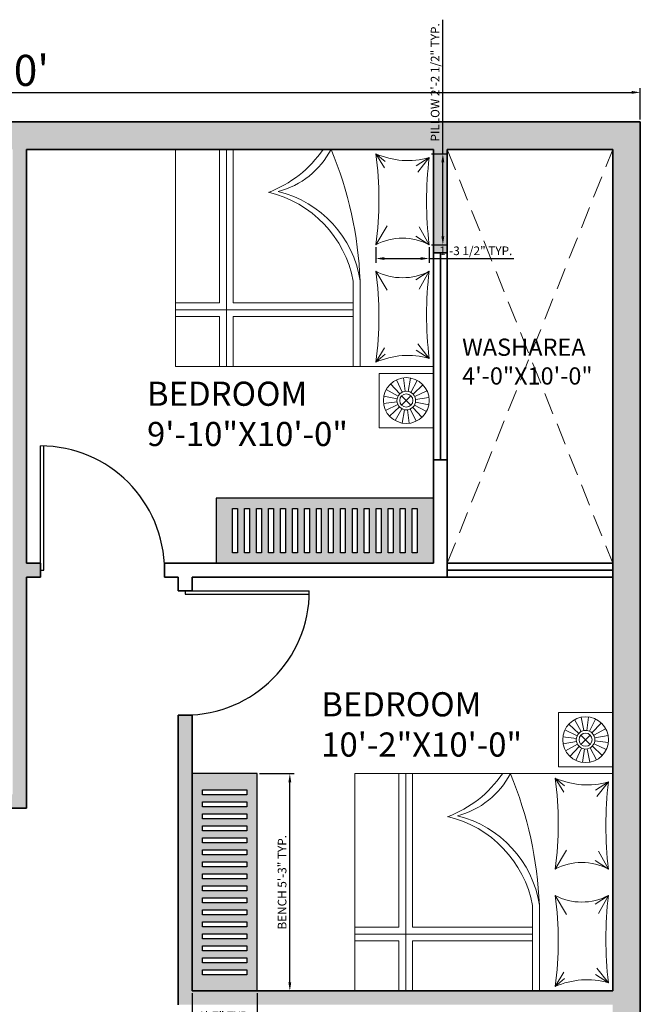
# Model space of a CAD drawing. Units: inches. Extents: x 1566 to 2546, y 1087 to 2705.
# Tile 23 of 27: x 2278 to 2458, y 1529 to 1814. Entities that reach past the tile are written whole.
import ezdxf

# ---------------------------------------------------------------- set-up
doc = ezdxf.new("R2010")
doc.units = ezdxf.units.IN
doc.linetypes.add('DASHED', pattern=[19.05, 12.7, -6.35])
for name, color, linetype, lineweight in [('A-ANNO-DIMS', 2, 'Continuous', 18), ('A-AREA-IDEN', 7, 'Continuous', 18), ('A-DOOR', 4, 'Continuous', 25), ('A-FLOR-OVHD', 8, 'DASHED', 18), ('A-FURN', 8, 'Continuous', 18), ('A-WALL', 7, 'Continuous', 35), ('A-WALL-PATT', 8, 'Continuous', 13)]:
    doc.layers.add(name, color=color, linetype=linetype, lineweight=lineweight)
doc.layers.add('MESA', color=7, linetype='Continuous')
doc.styles.get("Standard").update_dxf_attribs({"font": 'arial.ttf'})
doc.dimstyles.new('ISO-25', dxfattribs={"dimtxt": 2.5, "dimasz": 2.5, "dimexe": 1.25, "dimexo": 0.625, "dimtad": 1, "dimtxsty": 'Standard', "dimcen": 2.5, "dimadec": 0, "dimazin": 0, "dimtfac": 1, "dimtmove": 0, "dimatfit": 3, "dimfxl": 1, "dimarcsym": 0})

# ---------------------------------------------------------------- blocks, each defined once
blk = doc.blocks.new('*D2')
at = {"layer": 'A-ANNO-DIMS', "color": 0, "lineweight": -2, "transparency": 16777216}
for p, q in [((2098.29, 1785.06), (2098.29, 1794.2)), ((2100.79, 1792.95), (2455.79, 1792.95)), ((2458.29, 1785.06), (2458.29, 1794.2))]:
    blk.add_line(p, q, dxfattribs=at)
at = {"layer": 'A-ANNO-DIMS', "color": 0, "transparency": 16777216}
for points in [[(2100.79, 1793.37), (2100.79, 1792.53), (2098.29, 1792.95)], [(2455.79, 1793.37), (2455.79, 1792.53), (2458.29, 1792.95)]]:
    blk.add_solid(points, dxfattribs=at)
at = {"layer": 'Defpoints', "color": 0, "transparency": 16777216}
for p in [(2458.29, 1792.95), (2098.29, 1784.43), (2458.29, 1784.43)]:
    blk.add_point(p, dxfattribs=at)
at = {"layer": 'A-ANNO-DIMS', "color": 0, "transparency": 16777216, "insert": (2278.29, 1798.17), "char_height": 9, "attachment_point": 5}
blk.add_mtext("30'", dxfattribs=at)
blk = doc.blocks.new('d1')
for p, q in [((3297.32, 1596.93), (3297.32, 1632.93)), ((3298.32, 1596.93), (3298.32, 1632.93)), ((3297.32, 1596.93), (3298.32, 1596.93))]:
    blk.add_line(p, q)
at = {"ltscale": 0.3}
blk.add_arc((3297.32, 1596.93), 36, 0, 90, dxfattribs=at)
blk = doc.blocks.new('Banco Lintz')
at = {"layer": 'MESA', "ltscale": 0.05}
h = blk.add_hatch(color=256, dxfattribs=at)
h.dxf.hatch_style = 1
h.set_gradient(color1=(138, 84, 66), color2=(0, 0, 0), one_color=1, name='INVCYLINDER')
h.paths.add_polyline_path([(0.48, 0), (0, 0), (0, -1.6), (0.48, -1.6)])
h.paths.add_polyline_path([(0.4034, -0.5091), (0.0766, -0.5091), (0.0766, -0.4724), (0.4034, -0.4724)], flags=16)
h.paths.add_polyline_path([(0.4034, -0.5608), (0.4034, -0.5974), (0.0766, -0.5974), (0.0766, -0.5608)], flags=16)
h.paths.add_polyline_path([(0.4034, -0.4207), (0.0766, -0.4207), (0.0766, -0.384), (0.4034, -0.384)], flags=16)
h.paths.add_polyline_path([(0.4034, -0.6491), (0.4034, -0.6858), (0.0766, -0.6858), (0.0766, -0.6491)], flags=16)
h.paths.add_polyline_path([(0.4034, -0.3323), (0.0766, -0.3323), (0.0766, -0.2957), (0.4034, -0.2957)], flags=16)
h.paths.add_polyline_path([(0.4034, -0.7375), (0.4034, -0.7741), (0.0766, -0.7741), (0.0766, -0.7375)], flags=16)
h.paths.add_polyline_path([(0.4034, -0.244), (0.0766, -0.244), (0.0766, -0.2073), (0.4034, -0.2073)], flags=16)
h.paths.add_polyline_path([(0.4034, -0.8259), (0.4034, -0.8625), (0.0766, -0.8625), (0.0766, -0.8259)], flags=16)
h.paths.add_polyline_path([(0.4034, -0.1556), (0.0766, -0.1556), (0.0766, -0.119), (0.4034, -0.119)], flags=16)
h.paths.add_polyline_path([(0.4034, -0.9142), (0.4034, -0.9509), (0.0766, -0.9509), (0.0766, -0.9142)], flags=16)
h.paths.add_polyline_path([(0.4034, -1.0026), (0.4034, -1.0392), (0.0766, -1.0392), (0.0766, -1.0026)], flags=16)
h.paths.add_polyline_path([(0.4034, -1.0909), (0.4034, -1.1276), (0.0766, -1.1276), (0.0766, -1.0909)], flags=16)
h.paths.add_polyline_path([(0.4034, -1.1793), (0.4034, -1.216), (0.0766, -1.216), (0.0766, -1.1793)], flags=16)
h.paths.add_polyline_path([(0.4034, -1.2677), (0.4034, -1.3043), (0.0766, -1.3043), (0.0766, -1.2677)], flags=16)
h.paths.add_polyline_path([(0.4034, -1.356), (0.4034, -1.3927), (0.0766, -1.3927), (0.0766, -1.356)], flags=16)
h.paths.add_polyline_path([(0.4034, -1.4444), (0.4034, -1.481), (0.0766, -1.481), (0.0766, -1.4444)], flags=16)
for points in [[(0, -1.6), (0.48, -1.6), (0.48, 0), (0, 0)], [(0.0766, -0.119), (0.4034, -0.119), (0.4034, -0.1556), (0.0766, -0.1556)], [(0.0766, -0.2073), (0.4034, -0.2073), (0.4034, -0.244), (0.0766, -0.244)], [(0.0766, -0.2957), (0.4034, -0.2957), (0.4034, -0.3323), (0.0766, -0.3323)], [(0.0766, -0.384), (0.4034, -0.384), (0.4034, -0.4207), (0.0766, -0.4207)], [(0.0766, -0.4724), (0.4034, -0.4724), (0.4034, -0.5091), (0.0766, -0.5091)], [(0.0766, -0.5608), (0.4034, -0.5608), (0.4034, -0.5974), (0.0766, -0.5974)], [(0.0766, -0.6491), (0.4034, -0.6491), (0.4034, -0.6858), (0.0766, -0.6858)], [(0.0766, -0.7375), (0.4034, -0.7375), (0.4034, -0.7741), (0.0766, -0.7741)], [(0.0766, -0.8259), (0.4034, -0.8259), (0.4034, -0.8625), (0.0766, -0.8625)], [(0.0766, -0.9142), (0.4034, -0.9142), (0.4034, -0.9509), (0.0766, -0.9509)], [(0.0766, -1.0026), (0.4034, -1.0026), (0.4034, -1.0392), (0.0766, -1.0392)], [(0.0766, -1.0909), (0.4034, -1.0909), (0.4034, -1.1276), (0.0766, -1.1276)], [(0.0766, -1.1793), (0.4034, -1.1793), (0.4034, -1.216), (0.0766, -1.216)], [(0.0766, -1.2677), (0.4034, -1.2677), (0.4034, -1.3043), (0.0766, -1.3043)], [(0.0766, -1.356), (0.4034, -1.356), (0.4034, -1.3927), (0.0766, -1.3927)], [(0.0766, -1.4444), (0.4034, -1.4444), (0.4034, -1.481), (0.0766, -1.481)]]:
    blk.add_lwpolyline(points, close=True, dxfattribs=at)
blk = doc.blocks.new('PILLOW')
for p, q in [((0, 26.42), (2.52, 22.29)), ((0, 26.42), (2.72, 24.12)), ((15.48, 25.29), (11.7, 22.89)), ((15.48, 25.29), (12.15, 21.04)), ((0, 0), (3.27, 5.54)), ((15.48, 0), (12.59, 5.2)), ((15.48, 0), (11.65, 2.52))]:
    blk.add_line(p, q)
for points in [[(0, 26.42, -0.069628), (0, 0)], [(0, 26.42, 0.175461), (15.48, 25.29)], [(15.48, 25.29, 0.059544), (15.48, 0)], [(0, 0, -0.248743), (15.48, 0)]]:
    blk.add_lwpolyline(points, format="xyb")
blk = doc.blocks.new('*D41')
at = {"layer": 'A-ANNO-DIMS', "color": 0, "lineweight": -2, "transparency": 16777216}
for p, q in [((2347.81, 1595.43), (2357.89, 1595.43)), ((2356.64, 1534.93), (2356.64, 1592.93)), ((2347.81, 1532.43), (2357.89, 1532.43))]:
    blk.add_line(p, q, dxfattribs=at)
at = {"layer": 'A-ANNO-DIMS', "color": 0, "transparency": 16777216}
for points in [[(2356.22, 1592.93), (2357.05, 1592.93), (2356.64, 1595.43)], [(2356.22, 1534.93), (2357.05, 1534.93), (2356.64, 1532.43)]]:
    blk.add_solid(points, dxfattribs=at)
at = {"layer": 'Defpoints', "color": 0, "transparency": 16777216}
for p in [(2347.19, 1595.43), (2356.64, 1595.43), (2347.19, 1532.43)]:
    blk.add_point(p, dxfattribs=at)
at = {"layer": 'A-ANNO-DIMS', "color": 0, "transparency": 16777216, "insert": (2354.72, 1563.93), "char_height": 2.5, "attachment_point": 5, "rotation": 90}
blk.add_mtext('BENCH 5\'-3" TYP.', dxfattribs=at)
blk = doc.blocks.new('*D42')
at = {"layer": 'A-ANNO-DIMS', "color": 0, "lineweight": -2, "transparency": 16777216}
for p, q in [((2328.29, 1531.81), (2328.29, 1521.73)), ((2347.19, 1531.81), (2347.19, 1521.73)), ((2330.79, 1522.98), (2344.69, 1522.98))]:
    blk.add_line(p, q, dxfattribs=at)
at = {"layer": 'A-ANNO-DIMS', "color": 0, "transparency": 16777216}
for points in [[(2330.79, 1523.4), (2330.79, 1522.57), (2328.29, 1522.98)], [(2344.69, 1523.4), (2344.69, 1522.57), (2347.19, 1522.98)]]:
    blk.add_solid(points, dxfattribs=at)
at = {"layer": 'Defpoints', "color": 0, "transparency": 16777216}
for p in [(2328.29, 1532.43), (2347.19, 1532.43), (2347.19, 1522.98)]:
    blk.add_point(p, dxfattribs=at)
at = {"layer": 'A-ANNO-DIMS', "color": 0, "transparency": 16777216, "insert": (2337.74, 1524.87), "char_height": 2.5, "attachment_point": 5}
blk.add_mtext('1\'-7" TYP.', dxfattribs=at)
blk = doc.blocks.new('*D45')
at = {"layer": 'A-ANNO-DIMS', "color": 0, "lineweight": -2, "transparency": 16777216}
for p, q in [((2401.02, 1775.17), (2401.02, 1814.03)), ((2397.68, 1775.17), (2402.27, 1775.17)), ((2401.02, 1751.25), (2401.02, 1772.67)), ((2397.68, 1748.75), (2402.27, 1748.75))]:
    blk.add_line(p, q, dxfattribs=at)
at = {"layer": 'A-ANNO-DIMS', "color": 0, "transparency": 16777216}
for points in [[(2400.6, 1772.67), (2401.44, 1772.67), (2401.02, 1775.17)], [(2400.6, 1751.25), (2401.44, 1751.25), (2401.02, 1748.75)]]:
    blk.add_solid(points, dxfattribs=at)
at = {"layer": 'Defpoints', "color": 0, "transparency": 16777216}
for p in [(2397.06, 1775.17), (2401.02, 1775.17), (2397.06, 1748.75)]:
    blk.add_point(p, dxfattribs=at)
at = {"layer": 'A-ANNO-DIMS', "color": 0, "transparency": 16777216, "insert": (2399.1, 1795.85), "char_height": 2.5, "attachment_point": 5, "rotation": 90}
blk.add_mtext('PILLOW 2\'-2 1/2" TYP.', dxfattribs=at)
blk = doc.blocks.new('*D46')
at = {"layer": 'A-ANNO-DIMS', "color": 0, "lineweight": -2, "transparency": 16777216}
for p, q in [((2381.57, 1748.12), (2381.57, 1743.53)), ((2397.06, 1748.12), (2397.06, 1743.53)), ((2384.07, 1744.78), (2394.56, 1744.78)), ((2397.06, 1744.78), (2421.63, 1744.78))]:
    blk.add_line(p, q, dxfattribs=at)
at = {"layer": 'A-ANNO-DIMS', "color": 0, "transparency": 16777216}
for points in [[(2384.07, 1745.2), (2384.07, 1744.37), (2381.57, 1744.78)], [(2394.56, 1745.2), (2394.56, 1744.37), (2397.06, 1744.78)]]:
    blk.add_solid(points, dxfattribs=at)
at = {"layer": 'Defpoints', "color": 0, "transparency": 16777216}
for p in [(2381.57, 1748.75), (2397.06, 1748.75), (2397.06, 1744.78)]:
    blk.add_point(p, dxfattribs=at)
at = {"layer": 'A-ANNO-DIMS', "color": 0, "transparency": 16777216, "insert": (2410.59, 1746.7), "char_height": 2.5, "attachment_point": 5}
blk.add_mtext('1\'-3 1/2" TYP.', dxfattribs=at)

msp = doc.modelspace()

# ---------------------------------------------------------------- hatches: boundary and pattern name
at = {"layer": 'A-WALL-PATT'}
h = msp.add_hatch(color=256, dxfattribs=at)
h.dxf.hatch_style = 1
h.paths.add_polyline_path([(2106.29, 1385.43), (2228.29, 1385.43), (2228.29, 1391.43), (2224.29, 1391.43), (2224.29, 1389.43), (2106.29, 1389.43), (2106.29, 1402.93), (2098.29, 1402.93), (2098.29, 1343.43), (2106.29, 1343.43), (2106.29, 1347.74)], flags=17)
h.paths.add_polyline_path([(2106.29, 1259.43), (2098.29, 1259.43), (2098.29, 1209.43), (2155.29, 1209.43), (2155.29, 1217.43), (2143.41, 1217.43), (2106.29, 1217.43)], flags=17)
h.paths.add_polyline_path([(2334.29, 1217.43), (2280.29, 1217.43), (2280.29, 1389.43), (2284.29, 1389.43), (2284.29, 1391.43), (2284.29, 1393.43), (2276.29, 1393.43), (2276.29, 1217.43), (2227.29, 1217.43), (2227.29, 1209.43), (2334.29, 1209.43)], flags=17)
h.paths.add_polyline_path([(2106.29, 1486.43), (2098.29, 1486.43), (2098.29, 1460.88), (2099.11, 1461.64), (2100.44, 1462.65), (2101.57, 1463.26), (2099.97, 1460.62), (2098.29, 1458.1), (2098.29, 1456.93), (2100.35, 1456.93), (2100.77, 1457.12), (2103.56, 1457.95), (2106.29, 1458.4), (2106.29, 1470.43), (2224.29, 1470.43), (2224.29, 1427.43), (2228.29, 1427.43), (2228.29, 1474.43), (2192.29, 1474.43), (2192.29, 1476.43), (2188.29, 1476.43), (2188.29, 1474.43), (2106.29, 1474.43)], flags=17)
h.paths.add_polyline_path([(2106.29, 1585.43), (2192.29, 1585.43), (2192.29, 1589.43), (2098.29, 1589.43), (2098.29, 1573.93), (2106.29, 1573.93)], flags=17)
h.paths.add_polyline_path([(2228.29, 1585.43), (2232.29, 1585.43), (2232.29, 1589.43), (2224.29, 1589.43), (2222.29, 1589.43), (2222.29, 1585.43), (2224.29, 1585.43), (2224.29, 1532.43), (2106.29, 1532.43), (2106.29, 1543.93), (2098.29, 1543.93), (2098.29, 1516.43), (2106.29, 1516.43), (2106.29, 1528.43), (2188.29, 1528.43), (2188.29, 1506.43), (2192.29, 1506.43), (2192.29, 1528.43), (2224.29, 1528.43), (2224.29, 1506.43), (2228.29, 1506.43)], flags=17)
h.paths.add_polyline_path([(2106.29, 1680.43), (2098.29, 1680.43), (2098.29, 1625.43), (2106.29, 1625.43)], flags=17)
h.paths.add_polyline_path([(2458.29, 1784.43), (2098.29, 1784.43), (2098.29, 1776.43), (2276.29, 1776.43), (2276.29, 1589.43), (2268.29, 1589.43), (2268.29, 1585.43), (2280.29, 1585.43), (2280.29, 1652.43), (2284.29, 1652.43), (2284.29, 1656.43), (2280.29, 1656.43), (2280.29, 1776.43), (2398.29, 1776.43), (2398.29, 1746.43), (2402.29, 1746.43), (2402.29, 1776.43), (2450.29, 1776.43), (2450.29, 1532.43), (2375.49, 1532.43), (2328.29, 1532.43), (2328.29, 1612.43), (2324.29, 1612.43), (2324.29, 1528.43), (2450.29, 1528.43), (2450.29, 1447.43), (2291.29, 1447.43), (2291.29, 1443.43), (2324.29, 1443.43), (2324.29, 1393.43), (2320.29, 1393.43), (2320.29, 1389.43), (2330.29, 1389.43), (2330.29, 1393.43), (2328.29, 1393.43), (2328.29, 1443.43), (2412.29, 1443.43), (2412.29, 1433.43), (2416.29, 1433.43), (2416.29, 1443.43), (2450.29, 1443.43), (2450.29, 1393.43), (2416.29, 1393.43), (2416.29, 1403.43), (2412.29, 1403.43), (2412.29, 1393.43), (2360.29, 1393.43), (2360.29, 1389.43), (2450.29, 1389.43), (2450.29, 1217.43), (2396.29, 1217.43), (2396.29, 1209.43), (2450.29, 1209.43), (2450.29, 1136.43), (2458.29, 1136.43)])

# ---------------------------------------------------------------- linework, layer by layer
at = {"layer": 'A-FLOR-OVHD', "ltscale": 0.5}
for p, q in [((2402.29, 1776.43), (2450.29, 1656.43)), ((2402.29, 1656.43), (2450.29, 1776.43))]:
    msp.add_line(p, q, dxfattribs=at)
at = {"layer": 'A-FURN'}
for p, q in [((2336.28, 1731.91), (2336.28, 1776.43)), ((2338.25, 1776.43), (2338.25, 1713.44)), ((2340.21, 1731.91), (2340.21, 1776.43)), ((2398.29, 1776.43), (2398.29, 1695.72)), ((2375.04, 1713.44), (2375.04, 1738.2)), ((2323.49, 1731.91), (2336.28, 1731.91)), ((2340.21, 1731.91), (2375.04, 1731.91)), ((2323.49, 1729.94), (2375.04, 1729.94)), ((2323.49, 1727.97), (2336.28, 1727.97)), ((2336.28, 1713.44), (2336.28, 1727.97)), ((2340.21, 1727.97), (2375.04, 1727.97)), ((2340.21, 1713.44), (2340.21, 1727.97)), ((2382.54, 1695.72), (2382.54, 1711.47)), ((2382.54, 1711.47), (2398.29, 1711.47)), ((2390.07, 1706.28), (2389.57, 1710.18)), ((2390.92, 1706.25), (2391.65, 1710.12)), ((2388.56, 1705.56), (2385.86, 1708.43)), ((2389.26, 1706.04), (2387.58, 1709.6)), ((2391.71, 1705.97), (2393.6, 1709.42)), ((2392.38, 1705.45), (2395.25, 1708.15)), ((2387.76, 1704.1), (2383.89, 1704.83)), ((2388.05, 1704.9), (2384.59, 1706.79)), ((2389.06, 1704.95), (2391.77, 1702.25)), ((2389.06, 1702.25), (2391.77, 1704.95)), ((2392.86, 1704.75), (2396.42, 1706.43)), ((2393.09, 1703.94), (2397, 1704.44)), ((2387.74, 1703.26), (2383.83, 1702.76)), ((2387.97, 1702.45), (2384.41, 1700.76)), ((2388.45, 1701.75), (2385.58, 1699.05)), ((2392.27, 1701.63), (2394.97, 1698.77)), ((2392.78, 1702.3), (2396.24, 1700.41)), ((2393.07, 1703.1), (2396.94, 1702.36)), ((2389.12, 1701.23), (2387.23, 1697.78)), ((2389.91, 1700.95), (2389.18, 1697.08)), ((2390.76, 1700.92), (2391.26, 1697.01)), ((2391.57, 1701.16), (2393.25, 1697.6)), ((2398.29, 1695.72), (2382.54, 1695.72)), ((2434.54, 1613.14), (2434.54, 1597.39)), ((2450.29, 1613.14), (2434.54, 1613.14)), ((2450.29, 1597.39), (2450.29, 1613.14)), ((2441.12, 1607.64), (2439.23, 1611.09)), ((2441.91, 1607.92), (2441.18, 1611.79)), ((2442.76, 1607.95), (2443.26, 1611.85)), ((2443.57, 1607.71), (2445.25, 1611.27)), ((2444.27, 1607.23), (2446.97, 1610.1)), ((2439.97, 1606.42), (2436.41, 1608.1)), ((2440.45, 1607.12), (2437.58, 1609.82)), ((2444.78, 1606.56), (2448.24, 1608.46)), ((2439.74, 1605.61), (2435.83, 1606.11)), ((2439.76, 1604.77), (2435.89, 1604.03)), ((2441.06, 1603.92), (2443.77, 1606.62)), ((2441.06, 1606.62), (2443.77, 1603.92)), ((2445.07, 1605.77), (2448.94, 1606.5)), ((2445.09, 1604.93), (2449, 1604.43)), ((2440.05, 1603.97), (2436.59, 1602.08)), ((2440.56, 1603.3), (2437.86, 1600.44)), ((2441.26, 1602.83), (2439.58, 1599.27)), ((2442.07, 1602.59), (2441.57, 1598.68)), ((2442.92, 1602.61), (2443.65, 1598.75)), ((2443.71, 1602.9), (2445.6, 1599.45)), ((2444.38, 1603.42), (2447.25, 1600.72)), ((2444.86, 1604.11), (2448.42, 1602.43)), ((2434.54, 1597.39), (2450.29, 1597.39)), ((2388.28, 1550.9), (2388.28, 1595.43)), ((2390.25, 1595.43), (2390.25, 1532.43)), ((2392.21, 1550.9), (2392.21, 1595.43)), ((2450.29, 1595.43), (2450.29, 1532.43)), ((2427.04, 1532.43), (2427.04, 1557.19)), ((2375.49, 1550.9), (2388.28, 1550.9)), ((2392.21, 1550.9), (2427.04, 1550.9)), ((2375.49, 1548.93), (2427.04, 1548.93)), ((2375.49, 1546.96), (2388.28, 1546.96)), ((2388.28, 1532.43), (2388.28, 1546.96)), ((2392.21, 1546.96), (2427.04, 1546.96)), ((2392.21, 1532.43), (2392.21, 1546.96))]:
    msp.add_line(p, q, dxfattribs=at)
for points in [[(2398.29, 1776.43), (2323.49, 1776.43), (2323.49, 1713.44), (2398.29, 1713.44)], [(2450.29, 1595.43), (2375.49, 1595.43), (2375.49, 1532.43), (2450.29, 1532.43)]]:
    msp.add_lwpolyline(points, dxfattribs=at)
for points in [[(2377.01, 1713.44), (2377.01, 1738.35, 0.303651), (2353.28, 1764.2, 0.210515), (2368.61, 1776.43)], [(2429.01, 1532.43), (2429.01, 1557.34, 0.303651), (2405.28, 1583.19, 0.210515), (2420.61, 1595.43)]]:
    msp.add_lwpolyline(points, format="xyb", dxfattribs=at)
for centre, radius in [((2390.42, 1703.6), 6.64), ((2390.42, 1703.6), 2.7), ((2390.42, 1703.6), 1.91), ((2442.42, 1605.27), 6.64), ((2442.42, 1605.27), 2.7), ((2442.42, 1605.27), 1.91)]:
    msp.add_circle(centre, radius, dxfattribs=at)
for centre, radius, start, end in [((2338.87, 1794.99), 33.1, 290.4105, 325.8901), ((2266.04, 1733.86), 111.06, 2.3174, 22.5397), ((2343.01, 1732.26), 32.57, 10.5107, 76.872), ((2390.87, 1613.98), 33.1, 290.4105, 325.8901), ((2318.04, 1552.85), 111.06, 2.3174, 22.5397), ((2395.01, 1551.25), 32.57, 10.5107, 76.872)]:
    msp.add_arc(centre, radius, start, end, dxfattribs=at)
at = {"layer": 'A-WALL'}
for p, q in [((2098.29, 1784.43), (2458.29, 1784.43)), ((2458.29, 1784.43), (2458.29, 1136.43)), ((2280.29, 1776.43), (2398.29, 1776.43)), ((2280.29, 1656.43), (2280.29, 1776.43)), ((2398.29, 1656.43), (2398.29, 1776.43)), ((2402.29, 1776.43), (2450.29, 1776.43)), ((2402.29, 1652.43), (2402.29, 1776.43)), ((2450.29, 1776.43), (2450.29, 1532.43)), ((2398.29, 1746.43), (2402.29, 1746.43)), ((2400.29, 1746.43), (2400.29, 1686.43)), ((2398.29, 1686.43), (2402.29, 1686.43)), ((2280.29, 1656.43), (2284.29, 1656.43)), ((2284.29, 1652.43), (2284.29, 1656.43)), ((2320.29, 1652.43), (2320.29, 1656.43)), ((2320.29, 1656.43), (2398.29, 1656.43)), ((2402.29, 1656.43), (2450.29, 1656.43)), ((2450.29, 1654.43), (2402.29, 1654.43)), ((2280.29, 1652.43), (2284.29, 1652.43)), ((2280.29, 1585.43), (2280.29, 1652.43)), ((2320.29, 1652.43), (2324.29, 1652.43)), ((2324.29, 1652.43), (2324.29, 1648.43)), ((2328.29, 1652.43), (2328.29, 1648.43)), ((2328.29, 1652.43), (2450.29, 1652.43)), ((2324.29, 1648.43), (2328.29, 1648.43)), ((2324.29, 1612.43), (2324.29, 1528.43)), ((2324.29, 1612.43), (2328.29, 1612.43)), ((2328.29, 1612.43), (2328.29, 1532.43)), ((2268.29, 1585.43), (2280.29, 1585.43)), ((2328.29, 1532.43), (2450.29, 1532.43))]:
    msp.add_line(p, q, dxfattribs=at)

# ---------------------------------------------------------------- block references
at = {"layer": 'A-DOOR'}
msp.add_blockref('d1', (-1013.03, 57.51), dxfattribs=at)
at = {"layer": 'A-DOOR', "rotation": 270}
msp.add_blockref('d1', (729.36, 4945.76), dxfattribs=at)
at = {"layer": 'A-FURN'}
for p in [(2381.57, 1748.75), (2433.57, 1567.74)]:
    msp.add_blockref('PILLOW', p, dxfattribs=at)
at = {"layer": 'A-FURN', "extrusion": (0, 0, -1), "zscale": -1, "rotation": 180}
for p in [(-2381.58, 1741.13), (-2433.57, 1560.12)]:
    msp.add_blockref('PILLOW', p, dxfattribs=at)
at = {"layer": 'A-FURN', "xscale": 39.3701, "yscale": 39.3701, "zscale": 39.3701, "rotation": 270}
msp.add_blockref('Banco Lintz', (2398.29, 1675.33), dxfattribs=at)
at = {"layer": 'A-FURN', "xscale": 39.3701, "yscale": 39.3701, "zscale": 39.3701}
msp.add_blockref('Banco Lintz', (2328.29, 1595.43), dxfattribs=at)

# ---------------------------------------------------------------- texts
at = {"layer": 'A-AREA-IDEN', "attachment_point": 1}
for s, insert, char_height in [('WASHAREA\\P4\'-0"X10\'-0"', (2406.61, 1721.57), 5), ('BEDROOM\\P9\'-10"X10\'-0"', (2315.22, 1709.08), 7), ('BEDROOM\\P10\'-2"X10\'-0"', (2365.74, 1619.04), 7)]:
    msp.add_mtext_dynamic_manual_height_columns(s, width=111.7553, gutter_width=12.5, heights=[0], dxfattribs=dict(at, insert=insert, char_height=char_height))

# ---------------------------------------------------------------- dimensions: what is measured, and where the dimension line sits
at = {"layer": 'A-ANNO-DIMS'}
for base, p1, p2, text, picture, middle in [((2401.02, 1775.17), (2397.06, 1748.75), (2397.06, 1775.17), 'PILLOW <> TYP.', '*D45', (2399.1, 1795.85)), ((2356.64, 1595.43), (2347.19, 1532.43), (2347.19, 1595.43), 'BENCH <> TYP.', '*D41', (2354.72, 1563.93))]:
    dim = msp.add_linear_dim(base=base, p1=p1, p2=p2, angle=90, text=text, dimstyle='ISO-25', override={"dimdec": 1, "dimrnd": 0, "dimzin": 1, "dimlunit": 4, "dimfrac": 2}, dxfattribs=at)
    dim.commit()
    dim.dimension.update_dxf_attribs({"geometry": picture, "text_midpoint": middle})
dim = msp.add_linear_dim(base=(2458.29, 1792.95), p1=(2098.29, 1784.43), p2=(2458.29, 1784.43), dimstyle='ISO-25', override={"dimtxt": 9, "dimdec": 1, "dimlunit": 3, "dimclrd": 0, "dimclre": 0, "dimclrt": 0, "dimtdec": 1, "dimtmove": 1}, dxfattribs=at)
dim.commit()
dim.dimension.update_dxf_attribs({"geometry": '*D2', "text_midpoint": (2278.29, 1798.17)})
for base, p1, p2, picture, middle in [((2397.06, 1744.78), (2381.57, 1748.75), (2397.06, 1748.75), '*D46', (2410.59, 1746.7)), ((2347.19, 1522.98), (2328.29, 1532.43), (2347.19, 1532.43), '*D42', (2337.74, 1524.87))]:
    dim = msp.add_linear_dim(base=base, p1=p1, p2=p2, text='<> TYP.', dimstyle='ISO-25', override={"dimdec": 1, "dimrnd": 0, "dimzin": 1, "dimlunit": 4, "dimfrac": 2}, dxfattribs=at)
    dim.commit()
    dim.dimension.update_dxf_attribs({"geometry": picture, "text_midpoint": middle})

doc.saveas('drawing.dxf')
